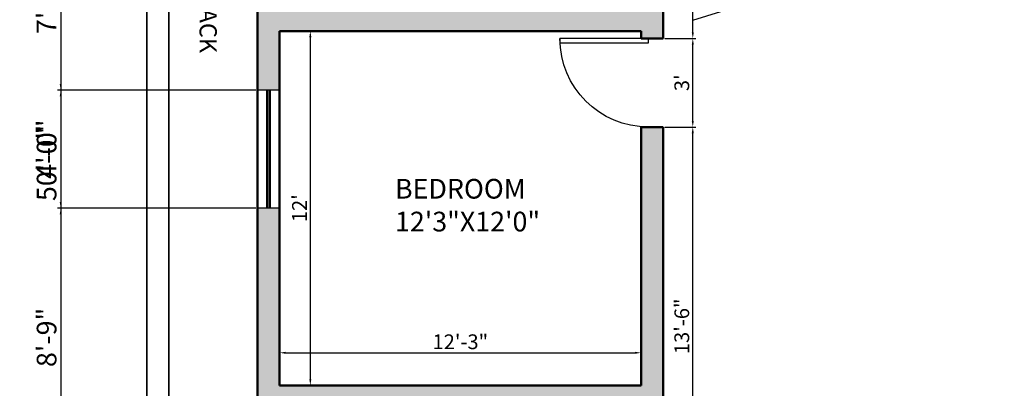
# Model space of a CAD drawing. Units: inches. Extents: x 2442 to 3851, y 589 to 2836.
# Tile 19 of 22: x 3157 to 3558, y 2400 to 2550. Entities that reach past the tile are written whole.
import ezdxf

# ---------------------------------------------------------------- set-up
doc = ezdxf.new("R2010")
doc.units = ezdxf.units.IN
for name, color, linetype, lineweight in [('A-ANNO-DIMS', 2, 'Continuous', 18), ('A-ANNO-TEXT', 7, 'Continuous', 18), ('A-AREA-IDEN', 7, 'Continuous', 18), ('A-DOOR', 4, 'Continuous', 25), ('A-GLAZ', 1, 'Continuous', 25), ('A-WALL', 7, 'Continuous', 50), ('A-WALL-PATT', 8, 'Continuous', 13), ('C-PROP', 7, 'Continuous', 35)]:
    doc.layers.add(name, color=color, linetype=linetype, lineweight=lineweight)
doc.styles.get("Standard").update_dxf_attribs({"font": 'arial.ttf'})
doc.dimstyles.new('ISO-25', dxfattribs={"dimtxt": 8, "dimasz": 2.5, "dimexe": 1.25, "dimexo": 0.625, "dimtad": 1, "dimlunit": 3, "dimtxsty": 'Standard', "dimcen": 2.5, "dimadec": 0, "dimazin": 0, "dimtfac": 1, "dimtmove": 0, "dimatfit": 3, "dimfxl": 1, "dimarcsym": 0})

# ---------------------------------------------------------------- blocks, each defined once
blk = doc.blocks.new('*U23')
for p, q in [((0, 0), (0, -6)), ((36, 0), (36, -6))]:
    blk.add_line(p, q)
blk.add_lwpolyline([(0, 0), (0, 36), (1.75, 36), (1.75, 0)], close=True)
blk.add_arc((0, 0), 36, 0, 90)
blk = doc.blocks.new('*D97')
at = {"layer": 'A-ANNO-DIMS', "color": 0, "lineweight": -2, "transparency": 16777216}
for p, q in [((3419.65, 2506.21), (3432.29, 2506.21)), ((3431.04, 2346.71), (3431.04, 2503.71)), ((3419.65, 2344.21), (3432.29, 2344.21))]:
    blk.add_line(p, q, dxfattribs=at)
at = {"layer": 'A-ANNO-DIMS', "color": 0, "transparency": 16777216}
for points in [[(3430.63, 2503.71), (3431.46, 2503.71), (3431.04, 2506.21)], [(3430.63, 2346.71), (3431.46, 2346.71), (3431.04, 2344.21)]]:
    blk.add_solid(points, dxfattribs=at)
at = {"layer": 'Defpoints', "color": 0, "transparency": 16777216}
for p in [(3419.02, 2506.21), (3431.04, 2506.21), (3419.02, 2344.21)]:
    blk.add_point(p, dxfattribs=at)
at = {"layer": 'A-ANNO-DIMS', "color": 0, "transparency": 16777216, "insert": (3427.35, 2425.21), "char_height": 6, "attachment_point": 5, "rotation": 90}
blk.add_mtext('13\'-6"', dxfattribs=at)
blk = doc.blocks.new('*D98')
at = {"layer": 'A-ANNO-DIMS', "color": 0, "lineweight": -2, "transparency": 16777216}
for p, q in [((3419.65, 2542.21), (3432.29, 2542.21)), ((3431.04, 2508.71), (3431.04, 2539.71)), ((3419.65, 2506.21), (3432.29, 2506.21))]:
    blk.add_line(p, q, dxfattribs=at)
at = {"layer": 'A-ANNO-DIMS', "color": 0, "transparency": 16777216}
for points in [[(3430.63, 2539.71), (3431.46, 2539.71), (3431.04, 2542.21)], [(3430.63, 2508.71), (3431.46, 2508.71), (3431.04, 2506.21)]]:
    blk.add_solid(points, dxfattribs=at)
at = {"layer": 'Defpoints', "color": 0, "transparency": 16777216}
for p in [(3419.02, 2542.21), (3431.04, 2542.21), (3419.02, 2506.21)]:
    blk.add_point(p, dxfattribs=at)
at = {"layer": 'A-ANNO-DIMS', "color": 0, "transparency": 16777216, "insert": (3427.35, 2524.21), "char_height": 6, "attachment_point": 5, "rotation": 90}
blk.add_mtext("3'", dxfattribs=at)
blk = doc.blocks.new('*D99')
at = {"layer": 'A-ANNO-DIMS', "color": 0, "lineweight": -2, "transparency": 16777216}
for p, q in [((3442.43, 2553.12), (3442.43, 2569.76)), ((3419.65, 2557.21), (3432.29, 2557.21)), ((3431.04, 2544.71), (3431.04, 2554.71)), ((3431.04, 2549.71), (3442.43, 2553.12)), ((3419.65, 2542.21), (3432.29, 2542.21))]:
    blk.add_line(p, q, dxfattribs=at)
at = {"layer": 'A-ANNO-DIMS', "color": 0, "transparency": 16777216}
for points in [[(3430.63, 2554.71), (3431.46, 2554.71), (3431.04, 2557.21)], [(3430.63, 2544.71), (3431.46, 2544.71), (3431.04, 2542.21)]]:
    blk.add_solid(points, dxfattribs=at)
at = {"layer": 'Defpoints', "color": 0, "transparency": 16777216}
for p in [(3419.02, 2557.21), (3431.04, 2557.21), (3419.02, 2542.21)]:
    blk.add_point(p, dxfattribs=at)
at = {"layer": 'A-ANNO-DIMS', "color": 0, "transparency": 16777216, "insert": (3438.74, 2561.44), "char_height": 6, "attachment_point": 5, "rotation": 90}
blk.add_mtext('1\'-3"', dxfattribs=at)
blk = doc.blocks.new('*D128')
at = {"layer": 'A-ANNO-DIMS', "color": 0, "lineweight": -2, "transparency": 16777216}
for p, q in [((3263.65, 2545.21), (3276.77, 2545.21)), ((3275.52, 2542.71), (3275.52, 2403.71)), ((3263.65, 2401.21), (3276.77, 2401.21))]:
    blk.add_line(p, q, dxfattribs=at)
at = {"layer": 'A-ANNO-DIMS', "color": 0, "transparency": 16777216}
for points in [[(3275.1, 2542.71), (3275.94, 2542.71), (3275.52, 2545.21)], [(3275.1, 2403.71), (3275.94, 2403.71), (3275.52, 2401.21)]]:
    blk.add_solid(points, dxfattribs=at)
at = {"layer": 'Defpoints', "color": 0, "transparency": 16777216}
for p in [(3263.02, 2545.21), (3263.02, 2401.21), (3275.52, 2401.21)]:
    blk.add_point(p, dxfattribs=at)
at = {"layer": 'A-ANNO-DIMS', "color": 0, "transparency": 16777216, "insert": (3271.88, 2473.21), "char_height": 6, "attachment_point": 5, "rotation": 90}
blk.add_mtext("12'", dxfattribs=at)
blk = doc.blocks.new('*D129')
at = {"layer": 'A-ANNO-DIMS', "color": 0, "lineweight": -2, "transparency": 16777216}
for p, q in [((3263.02, 2401.83), (3263.02, 2415.71)), ((3265.52, 2414.46), (3407.52, 2414.46)), ((3410.02, 2401.83), (3410.02, 2415.71))]:
    blk.add_line(p, q, dxfattribs=at)
at = {"layer": 'A-ANNO-DIMS', "color": 0, "transparency": 16777216}
for points in [[(3265.52, 2414.87), (3265.52, 2414.04), (3263.02, 2414.46)], [(3407.52, 2414.87), (3407.52, 2414.04), (3410.02, 2414.46)]]:
    blk.add_solid(points, dxfattribs=at)
at = {"layer": 'Defpoints', "color": 0, "transparency": 16777216}
for p in [(3410.02, 2414.46), (3263.02, 2401.21), (3410.02, 2401.21)]:
    blk.add_point(p, dxfattribs=at)
at = {"layer": 'A-ANNO-DIMS', "color": 0, "transparency": 16777216, "insert": (3336.52, 2418.15), "char_height": 6, "attachment_point": 5}
blk.add_mtext('12\'-3"', dxfattribs=at)
blk = doc.blocks.new('*D219')
at = {"layer": 'A-ANNO-DIMS', "color": 0, "lineweight": -2, "transparency": 16777216}
for p, q in [((3208.4, 2791.21), (3172.77, 2791.21)), ((3174.02, 2788.71), (3174.02, 2193.71)), ((3208.4, 2191.21), (3172.77, 2191.21))]:
    blk.add_line(p, q, dxfattribs=at)
at = {"layer": 'A-ANNO-DIMS', "color": 0, "transparency": 16777216}
for points in [[(3173.61, 2788.71), (3174.44, 2788.71), (3174.02, 2791.21)], [(3173.61, 2193.71), (3174.44, 2193.71), (3174.02, 2191.21)]]:
    blk.add_solid(points, dxfattribs=at)
at = {"layer": 'Defpoints', "color": 0, "transparency": 16777216}
for p in [(3209.02, 2791.21), (3174.02, 2191.21), (3209.02, 2191.21)]:
    blk.add_point(p, dxfattribs=at)
at = {"layer": 'A-ANNO-DIMS', "color": 0, "transparency": 16777216, "insert": (3169.31, 2491.21), "char_height": 8, "attachment_point": 5, "rotation": 90}
blk.add_mtext('50\'-0"', dxfattribs=at)
blk = doc.blocks.new('*D238')
at = {"layer": 'A-ANNO-DIMS', "color": 0, "lineweight": -2, "transparency": 16777216}
for p, q in [((3253.4, 2609.71), (3172.77, 2609.71)), ((3174.02, 2607.21), (3174.02, 2523.71)), ((3253.4, 2521.21), (3172.77, 2521.21))]:
    blk.add_line(p, q, dxfattribs=at)
at = {"layer": 'A-ANNO-DIMS', "color": 0, "transparency": 16777216}
for points in [[(3173.61, 2607.21), (3174.44, 2607.21), (3174.02, 2609.71)], [(3173.61, 2523.71), (3174.44, 2523.71), (3174.02, 2521.21)]]:
    blk.add_solid(points, dxfattribs=at)
at = {"layer": 'Defpoints', "color": 0, "transparency": 16777216}
for p in [(3254.02, 2609.71), (3174.02, 2521.21), (3254.02, 2521.21)]:
    blk.add_point(p, dxfattribs=at)
at = {"layer": 'A-ANNO-DIMS', "color": 0, "transparency": 16777216, "insert": (3169.26, 2565.46), "char_height": 8, "attachment_point": 5, "rotation": 90}
blk.add_mtext('7\'-4 1/2"', dxfattribs=at)
blk = doc.blocks.new('*D239')
at = {"layer": 'A-ANNO-DIMS', "color": 0, "lineweight": -2, "transparency": 16777216}
for p, q in [((3253.4, 2521.21), (3172.77, 2521.21)), ((3174.02, 2518.71), (3174.02, 2475.71)), ((3253.4, 2473.21), (3172.77, 2473.21))]:
    blk.add_line(p, q, dxfattribs=at)
at = {"layer": 'A-ANNO-DIMS', "color": 0, "transparency": 16777216}
for points in [[(3173.61, 2518.71), (3174.44, 2518.71), (3174.02, 2521.21)], [(3173.61, 2475.71), (3174.44, 2475.71), (3174.02, 2473.21)]]:
    blk.add_solid(points, dxfattribs=at)
at = {"layer": 'Defpoints', "color": 0, "transparency": 16777216}
for p in [(3254.02, 2521.21), (3174.02, 2473.21), (3254.02, 2473.21)]:
    blk.add_point(p, dxfattribs=at)
at = {"layer": 'A-ANNO-DIMS', "color": 0, "transparency": 16777216, "insert": (3169.31, 2497.21), "char_height": 8, "attachment_point": 5, "rotation": 90}
blk.add_mtext('4\'-0"', dxfattribs=at)
blk = doc.blocks.new('*D240')
at = {"layer": 'A-ANNO-DIMS', "color": 0, "lineweight": -2, "transparency": 16777216}
for p, q in [((3253.4, 2473.21), (3172.77, 2473.21)), ((3174.02, 2470.71), (3174.02, 2370.71)), ((3253.4, 2368.21), (3172.77, 2368.21))]:
    blk.add_line(p, q, dxfattribs=at)
at = {"layer": 'A-ANNO-DIMS', "color": 0, "transparency": 16777216}
for points in [[(3173.61, 2470.71), (3174.44, 2470.71), (3174.02, 2473.21)], [(3173.61, 2370.71), (3174.44, 2370.71), (3174.02, 2368.21)]]:
    blk.add_solid(points, dxfattribs=at)
at = {"layer": 'Defpoints', "color": 0, "transparency": 16777216}
for p in [(3254.02, 2473.21), (3174.02, 2368.21), (3254.02, 2368.21)]:
    blk.add_point(p, dxfattribs=at)
at = {"layer": 'A-ANNO-DIMS', "color": 0, "transparency": 16777216, "insert": (3169.31, 2420.71), "char_height": 8, "attachment_point": 5, "rotation": 90}
blk.add_mtext('8\'-9"', dxfattribs=at)

msp = doc.modelspace()

# ---------------------------------------------------------------- hatches: boundary and pattern name
at = {"layer": 'A-WALL-PATT'}
h = msp.add_hatch(color=256, dxfattribs=at)
h.dxf.hatch_style = 1
h.paths.add_polyline_path([(3356.024, 2713.208), (3356.024, 2719.208), (3356.024, 2722.208), (3254.024, 2722.208), (3254.024, 2657.708), (3263.024, 2657.708), (3263.024, 2713.208)])
h.paths.add_polyline_path([(3416.024, 2737.208), (3446.024, 2737.208), (3446.024, 2746.208), (3416.024, 2746.208), (3416.024, 2782.208), (3407.024, 2782.208), (3407.024, 2722.208), (3386.024, 2722.208), (3386.024, 2719.208), (3386.024, 2713.208), (3407.024, 2713.208), (3407.024, 2593.208), (3416.024, 2593.208), (3416.024, 2608.208), (3515.024, 2608.208), (3515.024, 2614.208), (3515.024, 2617.208), (3416.024, 2617.208)])
h.paths.add_polyline_path([(3563.024, 2737.208), (3566.024, 2737.208), (3566.024, 2746.208), (3512.024, 2746.208), (3512.024, 2737.208), (3554.024, 2737.208), (3554.024, 2617.208), (3551.024, 2617.208), (3551.024, 2614.208), (3551.024, 2608.208), (3554.024, 2608.208), (3554.024, 2554.208), (3566.024, 2554.208), (3566.024, 2560.208), (3566.024, 2563.208), (3563.024, 2563.208)])
h.paths.add_polyline_path([(3614.024, 2746.208), (3614.024, 2737.208), (3683.024, 2737.208), (3683.024, 2746.208)])
h.paths.add_polyline_path([(3755.024, 2737.208), (3755.024, 2665.208), (3764.024, 2665.208), (3764.024, 2746.208), (3731.024, 2746.208), (3731.024, 2737.208)])
h.paths.add_polyline_path([(3662.024, 2617.208), (3662.024, 2611.208), (3755.024, 2611.208), (3755.024, 2605.208), (3764.024, 2605.208), (3764.024, 2617.208)])
h.paths.add_polyline_path([(3755.024, 2554.208), (3755.024, 2548.208), (3764.024, 2548.208), (3764.024, 2569.208), (3755.024, 2569.208), (3755.024, 2563.208), (3677.024, 2563.208), (3677.024, 2581.208), (3671.024, 2581.208), (3671.024, 2563.208), (3611.024, 2563.208), (3611.024, 2611.208), (3632.024, 2611.208), (3632.024, 2617.208), (3605.024, 2617.208), (3605.024, 2563.208), (3602.024, 2563.208), (3602.024, 2554.208), (3653.024, 2554.208), (3653.024, 2536.208), (3659.024, 2536.208), (3659.024, 2554.208)])
h.paths.add_polyline_path([(3764.024, 2512.208), (3755.024, 2512.208), (3755.024, 2506.208), (3653.024, 2506.208), (3653.024, 2500.208), (3755.024, 2500.208), (3755.024, 2474.708), (3764.024, 2474.708)])
h.paths.add_polyline_path([(3608.024, 2392.208), (3764.024, 2392.208), (3764.024, 2426.708), (3755.024, 2426.708), (3755.024, 2401.208), (3608.024, 2401.208), (3608.024, 2461.208), (3599.024, 2461.208), (3599.024, 2353.208), (3608.024, 2353.208)])
h.paths.add_polyline_path([(3410.024, 2401.208), (3263.024, 2401.208), (3263.024, 2473.208), (3254.024, 2473.208), (3254.024, 2368.208), (3263.024, 2368.208), (3263.024, 2392.208), (3410.024, 2392.208), (3410.024, 2344.208), (3419.024, 2344.208), (3419.024, 2506.208), (3413.024, 2506.208), (3410.024, 2506.208)])
h.paths.add_polyline_path([(3263.024, 2609.708), (3254.024, 2609.708), (3254.024, 2521.208), (3263.024, 2521.208), (3263.024, 2545.208), (3410.024, 2545.208), (3410.024, 2542.208), (3413.024, 2542.208), (3419.024, 2542.208), (3419.024, 2557.208), (3407.024, 2557.208), (3407.024, 2554.208), (3263.024, 2554.208)])
h.paths.add_polyline_path([(3254.024, 2191.208), (3263.024, 2191.208), (3263.024, 2287.208), (3269.024, 2287.208), (3269.024, 2293.208), (3269.024, 2296.208), (3263.024, 2296.208), (3263.024, 2320.208), (3254.024, 2320.208)])
h.paths.add_polyline_path([(3419.024, 2296.208), (3386.024, 2296.208), (3386.024, 2287.208), (3410.024, 2287.208), (3410.024, 2191.208), (3419.024, 2191.208), (3419.024, 2248.208), (3449.024, 2248.208), (3449.024, 2257.208), (3419.024, 2257.208)])
h.paths.add_polyline_path([(3581.024, 2248.208), (3608.024, 2248.208), (3608.024, 2287.208), (3599.024, 2287.208), (3599.024, 2257.208), (3581.024, 2257.208)])
h.paths.add_polyline_path([(3491.024, 2248.208), (3515.024, 2248.208), (3515.024, 2257.208), (3491.024, 2257.208)])
h.paths.add_polyline_path([(3320.024, 2296.208), (3309.024, 2296.208), (3309.024, 2287.208), (3320.024, 2287.208)])
h.paths.add_polyline_path([(3282.007, 2631.263), (3387.059, 2631.263), (3387.059, 2661.678), (3282.007, 2661.678)], flags=9)
h.paths.add_polyline_path([(3511.253, 2214.916), (3571.545, 2214.916), (3571.545, 2229.862), (3511.253, 2229.862)], flags=9)
h.paths.add_polyline_path([(3777.335, 2589.915), (3777.335, 2529.623), (3792.281, 2529.623), (3792.281, 2589.915)], flags=9)
h.paths.add_polyline_path([(3558.97, 2754.629), (3619.262, 2754.629), (3619.262, 2769.575), (3558.97, 2769.575)], flags=9)
h.paths.add_polyline_path([(3314.979, 2749.318), (3377.263, 2749.318), (3377.263, 2779.733), (3314.979, 2779.733)], flags=9)
h.paths.add_polyline_path([(3624.453, 2577.252), (3671.045, 2577.252), (3671.045, 2600.063), (3624.453, 2600.063)], flags=25)
h.paths.add_polyline_path([(3701.15, 2577.252), (3744.07, 2577.252), (3744.07, 2600.063), (3701.15, 2600.063)], flags=25)
h.paths.add_polyline_path([(3689.533, 2518.545), (3731.868, 2518.545), (3731.868, 2541.356), (3689.533, 2541.356)], flags=9)
h.paths.add_polyline_path([(3629.196, 2666.979), (3693.452, 2666.979), (3693.452, 2697.394), (3629.196, 2697.394)], flags=9)
h.paths.add_polyline_path([(3441.284, 2669.891), (3505.54, 2669.891), (3505.54, 2700.306), (3441.284, 2700.306)], flags=25)
h.paths.add_polyline_path([(3306.565, 2459.233), (3370.821, 2459.233), (3370.821, 2489.648), (3306.565, 2489.648)], flags=25)
h.paths.add_polyline_path([(3307.889, 2320.733), (3387.355, 2320.733), (3387.355, 2351.148), (3307.889, 2351.148)], flags=9)
h.paths.add_polyline_path([(3452.987, 2372.794), (3554.971, 2372.794), (3554.971, 2403.208), (3452.987, 2403.208)], flags=9)

# ---------------------------------------------------------------- linework, layer by layer
at = {"layer": 'A-GLAZ'}
for p, q in [((3263.024, 2521.208), (3254.024, 2521.208)), ((3263.024, 2473.208), (3254.024, 2473.208))]:
    msp.add_line(p, q, dxfattribs=at)
at = {"layer": 'A-WALL'}
for p, q in [((3254.024, 2782.208), (3254.024, 2191.208)), ((3419.024, 2542.208), (3419.024, 2557.208)), ((3263.024, 2545.208), (3263.024, 2401.208)), ((3263.024, 2545.208), (3410.024, 2545.208)), ((3410.024, 2542.208), (3410.024, 2545.208)), ((3410.024, 2542.208), (3419.024, 2542.208)), ((3258.024, 2521.208), (3258.024, 2473.208)), ((3259.024, 2521.208), (3259.024, 2473.208)), ((3410.024, 2401.208), (3410.024, 2506.208)), ((3410.024, 2506.208), (3419.024, 2506.208)), ((3419.024, 2344.208), (3419.024, 2506.208)), ((3263.024, 2401.208), (3410.024, 2401.208))]:
    msp.add_line(p, q, dxfattribs=at)
at = {"layer": 'C-PROP'}
for points in [[(3809.024, 2191.208), (3809.024, 2791.208), (3209.024, 2791.208), (3209.024, 2191.208), (3809.024, 2191.208)], [(3800.024, 2200.208), (3800.024, 2782.208), (3218.024, 2782.208), (3218.024, 2200.208), (3254.024, 2200.208)]]:
    msp.add_lwpolyline(points, dxfattribs=at)

# ---------------------------------------------------------------- block references
at = {"layer": 'A-DOOR', "xscale": -1, "rotation": 90}
msp.add_blockref('*U23', (3413.024, 2542.208), dxfattribs=at)

# ---------------------------------------------------------------- texts
at = {"layer": 'A-ANNO-TEXT', "insert": (3237.481, 2587.746), "char_height": 7, "attachment_point": 1, "rotation": 270}
msp.add_mtext_dynamic_manual_height_columns("{\\fTimes New Roman|b0|i0|c0|p18;3' SETBACK}", width=79.56037, gutter_width=12.5, heights=[0], dxfattribs=at)
at = {"layer": 'A-AREA-IDEN', "insert": (3309.949, 2485.121), "char_height": 8, "attachment_point": 1}
msp.add_mtext_dynamic_manual_height_columns('{\\fTimes New Roman|b0|i0|c0|p18;BEDROOM\\P12\'3"X12\'0"}', width=110.76054, gutter_width=12.5, heights=[0], dxfattribs=at)

# ---------------------------------------------------------------- dimensions: what is measured, and where the dimension line sits
at = {"layer": 'A-ANNO-DIMS'}
for base, p1, p2, override, picture, middle in [((3174.024, 2191.208), (3209.024, 2791.208), (3209.024, 2191.208), {"dimdec": 1, "dimlfac": 1, "dimrnd": 0, "dimzin": 1, "dimdsep": 46, "dimlunit": 4, "dimfrac": 2}, '*D219', (3169.315, 2491.208)), ((3174.024, 2521.208), (3254.024, 2609.708), (3254.024, 2521.208), {"dimdec": 1, "dimlfac": 1, "dimrnd": 0, "dimzin": 1, "dimdsep": 46, "dimlunit": 4, "dimfrac": 2}, '*D238', (3169.263, 2565.458)), ((3431.044, 2557.208), (3419.024, 2542.208), (3419.024, 2557.208), {"dimtxt": 6, "dimclrd": 0, "dimclre": 0, "dimclrt": 0, "dimtmove": 1}, '*D99', (3438.737, 2553.748)), ((3275.52, 2401.208), (3263.024, 2545.208), (3263.024, 2401.208), {"dimtxt": 6, "dimclrd": 0, "dimclre": 0, "dimclrt": 0}, '*D128', (3271.883, 2473.208)), ((3431.044, 2542.208), (3419.024, 2506.208), (3419.024, 2542.208), {"dimtxt": 6, "dimclrd": 0, "dimclre": 0, "dimclrt": 0, "dimtmove": 1}, '*D98', (3427.353, 2524.208)), ((3174.024, 2473.208), (3254.024, 2521.208), (3254.024, 2473.208), {"dimdec": 1, "dimlfac": 1, "dimrnd": 0, "dimzin": 1, "dimdsep": 46, "dimlunit": 4, "dimfrac": 2}, '*D239', (3169.315, 2497.208)), ((3431.044, 2506.208), (3419.024, 2344.208), (3419.024, 2506.208), {"dimtxt": 6, "dimclrd": 0, "dimclre": 0, "dimclrt": 0, "dimtmove": 1}, '*D97', (3427.353, 2425.208)), ((3174.024, 2368.208), (3254.024, 2473.208), (3254.024, 2368.208), {"dimdec": 1, "dimlfac": 1, "dimrnd": 0, "dimzin": 1, "dimdsep": 46, "dimlunit": 4, "dimfrac": 2}, '*D240', (3169.315, 2420.708))]:
    dim = msp.add_linear_dim(base=base, p1=p1, p2=p2, angle=90, dimstyle='ISO-25', override=override, dxfattribs=at)
    dim.commit()
    dim.dimension.update_dxf_attribs({"geometry": picture, "text_midpoint": middle})
dim = msp.add_linear_dim(base=(3410.024, 2414.457), p1=(3263.024, 2401.208), p2=(3410.024, 2401.208), dimstyle='ISO-25', override={"dimtxt": 6, "dimclrd": 0, "dimclre": 0, "dimclrt": 0}, dxfattribs=at)
dim.commit()
dim.dimension.update_dxf_attribs({"geometry": '*D129', "text_midpoint": (3336.524, 2418.148)})

doc.saveas('drawing.dxf')
